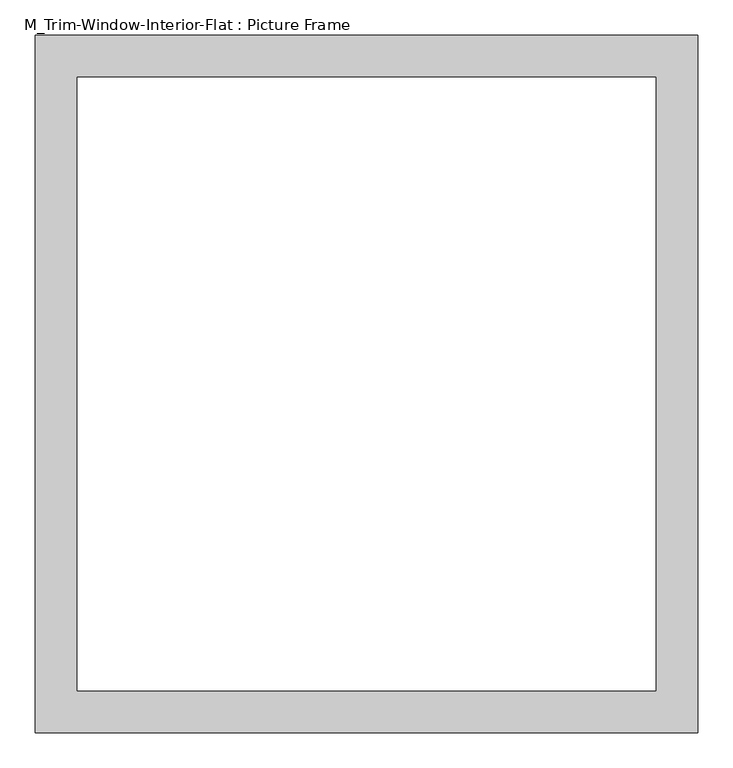
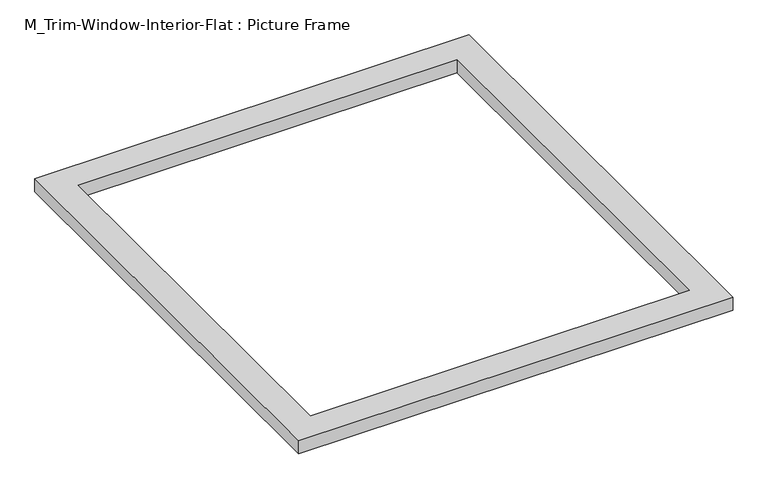
"""IFC4 building model written with IfcOpenShell, lengths in millimetres: proxy geometry, M_Trim-Window-Interior-Flat : Picture Frame."""

from ifc_helpers import new_model, si_unit, origin, origin_with_axes, place, context, project, spatial, polyline, outline, extrude, source, transform, mapped, element, save


def m_trim_window_interior_flat_picture_frame_6ca9b1f8(model_context):
    return source(origin(), model_context, "Body", "SweptSolid", [
        extrude(outline(polyline([(472.3, 47.3), (472.3, -947.3), (-472.3, -947.3), (-472.3, 47.3), (472.3, 47.3)]), holes=[polyline([(412.3, -12.7), (-412.3, -12.7), (-412.3, -887.3), (412.3, -887.3), (412.3, -12.7)])]), origin_with_axes(), (0.0, 0.0, 1.0), 30.0),
    ])


if __name__ == "__main__":
    model = new_model("IFC4")
    model_context = context("Model", 3, world=origin())
    ifc_project = project(units=[si_unit("LENGTHUNIT", "METRE", prefix="MILLI")], contexts=[model_context])
    site = spatial("IfcSite", under=ifc_project)
    building = spatial("IfcBuilding", under=site)
    placement = place(None, origin())
    m_trim_window_interior_flat_picture_frame_shape = m_trim_window_interior_flat_picture_frame_6ca9b1f8(model_context)
    element("IfcBuildingElementProxy", 1, Name="M_Trim-Window-Interior-Flat : Picture Frame", ObjectType="M_Trim-Window-Interior-Flat : Picture Frame", at=placement, inside=building, context=model_context, shape_type="MappedRepresentation", body=[
        mapped(m_trim_window_interior_flat_picture_frame_shape, transform((0.0, 0.0, 0.0), x_axis=(1.0, 0.0, 0.0), y_axis=(0.0, 1.0, 0.0), z_axis=(0.0, 0.0, 1.0))),
    ])
    save(model, "model.ifc")

# Revit data of these elements
# Type "M_Trim-Window-Interior-Flat : Picture Frame"
#   Trim Thickness_Picture Frame = 0.098425 ft
#   Trim Width = 0.19685 ft
#   Trim Thickness_with Sill = 0.065617 ft
#   Sill Thickness = 0.098425 ft
#   Opening Width [instance default] = 1.968504 ft
#   Opening Height [instance default] = 2.952756 ft
#   Default Elevation = 3.937008 ft
#   Sill = no
#   Picture Frame = yes
#   Trim Material [instance default] = none
# Element 1 (IfcBuildingElementProxy, "M_Trim-Window-Interior-Flat : Picture Frame")
#   Opening Width = 2.788714 ft
#   Trim Material = Wood - Stained
#   Materials on its faces: "Wood - Stained"
# Materials
#   "Wood - Stained": class "Wood", colour RGB 224 178 126, transparency 0, Cost = 0
